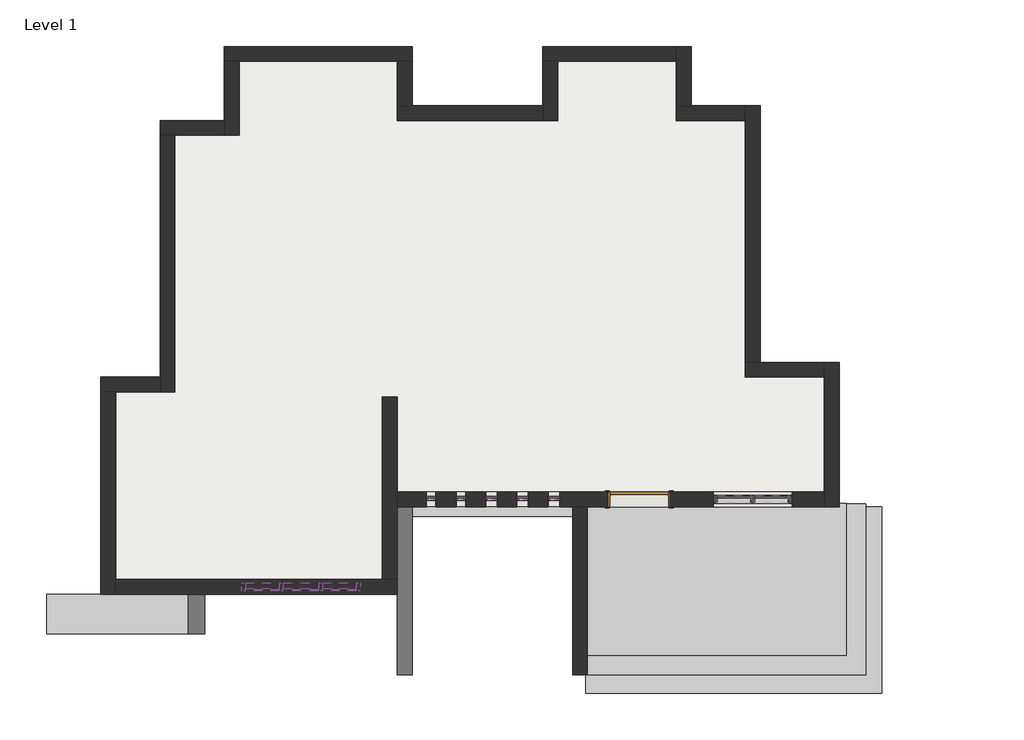
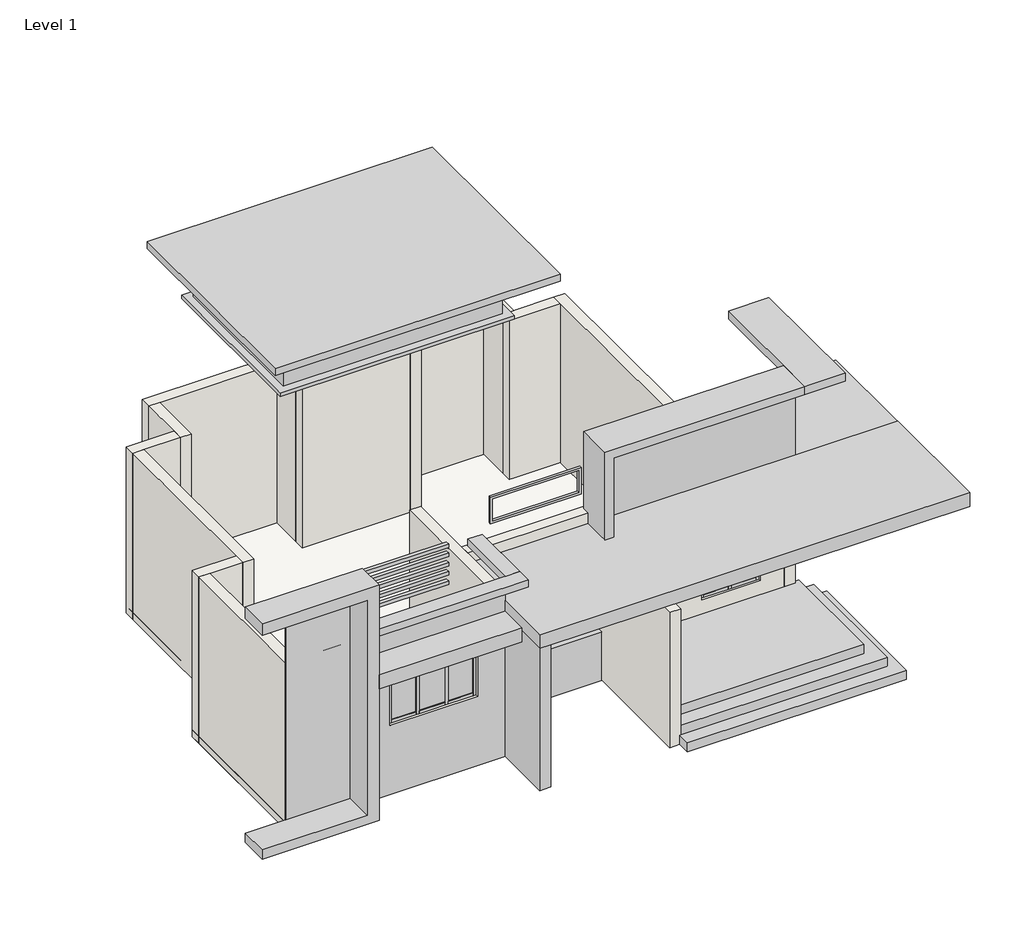
# One storey: 37 members, 19 walls, 10 plates, 1 door, 1 proxy, 1 slab.
"""IFC4 building model written with IfcOpenShell, lengths in millimetres."""

from ifc_helpers import new_model, si_unit, origin, origin_with_axes, place, context, project, spatial, polyline, outline, extrude, faceted_brep, transform, mapped, element, save
from components import generic_models_1_generic_models_1_dd7d6be2, door_e6f20f03, member_d2c643f7, member_0682bd88, member_4ec4fa50, member_0b7646a3, member_2b49869a, member_a980948f, member_75074519, member_d60e8053, member_2fae0574, system_panel_glazed_29dc7863, system_panel_glazed_ebf67a72, system_panel_glazed_1715a493, system_panel_glazed_fcede64b, system_panel_glazed_078fe0dd

model = new_model("IFC4")

# Units and contexts
model_context = context("Model", 3, world=origin())
ifc_project = project(units=[si_unit("LENGTHUNIT", "METRE", prefix="MILLI")], contexts=[model_context])

# Site, building, storey
site = spatial("IfcSite", under=ifc_project)
building = spatial("IfcBuilding", under=site)
storey = spatial("IfcBuildingStorey", under=building, Name="Level 1", Elevation=0.0)

# Proxy
placement = place(None, origin())
generic_models_1_generic_models_1_shape = generic_models_1_generic_models_1_dd7d6be2(model_context)
element("IfcBuildingElementProxy", 1, Name="Generic Models 1 : Generic Models 1", ObjectType="Generic Models 1 : Generic Models 1", at=placement, inside=storey, context=model_context, shape_type="MappedRepresentation", body=[
    mapped(generic_models_1_generic_models_1_shape, transform((0.0, 0.0, 0.0), x_axis=(1.0, 0.0, 0.0), y_axis=(0.0, 1.0, 0.0), z_axis=(0.0, 0.0, 1.0))),
])

# Door
door_shape = door_e6f20f03(model_context)
element("IfcDoor", 2, ObjectType="Door-Interior-Single-5_Panel_Vert-Wood : 3'6\" x 7'", at=placement, inside=storey, context=model_context, shape_type="MappedRepresentation", body=[
    mapped(door_shape, transform((1178.8071977, 2200.0207931, 609.6), x_axis=(-1.0, 0.0, 0.0), y_axis=(0.0, -1.0, 0.0), z_axis=(0.0, 0.0, 1.0))),
])

# Members
member_shape = member_d2c643f7(model_context)
element("IfcMember", 3, ObjectType="Rectangular Mullion : 1\" Square", at=placement, inside=storey, context=model_context, shape_type="MappedRepresentation", body=[
    mapped(member_shape, transform((-1983.4928023, 2196.8457931, 2975.2644013), x_axis=(0.0, 0.0, 1.0), y_axis=(0.0, -1.0, 0.0), z_axis=(1.0, 0.0, 0.0))),
])
element("IfcMember", 4, ObjectType="Rectangular Mullion : 1\" Square", at=placement, inside=storey, context=model_context, shape_type="MappedRepresentation", body=[
    mapped(member_shape, transform((-1519.9428023, 2196.8457931, 2975.2644013), x_axis=(0.0, 0.0, 1.0), y_axis=(0.0, -1.0, 0.0), z_axis=(1.0, 0.0, 0.0))),
])
element("IfcMember", 5, ObjectType="Rectangular Mullion : 1\" Square", at=placement, inside=storey, context=model_context, shape_type="MappedRepresentation", body=[
    mapped(member_shape, transform((-2085.0928023, 2196.8457931, 914.4), x_axis=(0.0, 0.0, -1.0), y_axis=(0.0, -1.0, 0.0), z_axis=(-1.0, 0.0, 0.0))),
])
element("IfcMember", 6, ObjectType="Rectangular Mullion : 1\" Square", at=placement, inside=storey, context=model_context, shape_type="MappedRepresentation", body=[
    mapped(member_shape, transform((-1621.5428023, 2196.8457931, 914.4), x_axis=(0.0, 0.0, -1.0), y_axis=(0.0, -1.0, 0.0), z_axis=(-1.0, 0.0, 0.0))),
])
member_2_shape = member_0682bd88(model_context)
element("IfcMember", 7, ObjectType="Rectangular Mullion : 1\" Square", at=placement, inside=storey, context=model_context, shape_type="MappedRepresentation", body=[
    mapped(member_2_shape, transform((-2110.4928023, 2196.8457931, 2975.2644013), x_axis=(-1.0, 0.0, 0.0), y_axis=(0.0, -1.0, 0.0), z_axis=(0.0, 0.0, 1.0))),
])
element("IfcMember", 8, ObjectType="Rectangular Mullion : 1\" Square", at=placement, inside=storey, context=model_context, shape_type="MappedRepresentation", body=[
    mapped(member_2_shape, transform((-1646.9428023, 2196.8457931, 2975.2644013), x_axis=(-1.0, 0.0, 0.0), y_axis=(0.0, -1.0, 0.0), z_axis=(0.0, 0.0, 1.0))),
])
element("IfcMember", 9, ObjectType="Rectangular Mullion : 1\" Square", at=placement, inside=storey, context=model_context, shape_type="MappedRepresentation", body=[
    mapped(member_2_shape, transform((-1189.7428023, 2196.8457931, 2975.2644013), x_axis=(-1.0, 0.0, 0.0), y_axis=(0.0, -1.0, 0.0), z_axis=(0.0, 0.0, 1.0))),
])
element("IfcMember", 10, ObjectType="Rectangular Mullion : 1\" Square", at=placement, inside=storey, context=model_context, shape_type="MappedRepresentation", body=[
    mapped(member_2_shape, transform((-707.1428023, 2196.8457931, 2975.2644013), x_axis=(-1.0, 0.0, 0.0), y_axis=(0.0, -1.0, 0.0), z_axis=(0.0, 0.0, 1.0))),
])
element("IfcMember", 11, ObjectType="Rectangular Mullion : 1\" Square", at=placement, inside=storey, context=model_context, shape_type="MappedRepresentation", body=[
    mapped(member_2_shape, transform((-224.5428023, 2196.8457931, 2975.2644013), x_axis=(-1.0, 0.0, 0.0), y_axis=(0.0, -1.0, 0.0), z_axis=(0.0, 0.0, 1.0))),
])
element("IfcMember", 12, ObjectType="Rectangular Mullion : 1\" Square", at=placement, inside=storey, context=model_context, shape_type="MappedRepresentation", body=[
    mapped(member_2_shape, transform((-1958.0928023, 2196.8457931, 914.4), x_axis=(1.0, 0.0, 0.0), y_axis=(0.0, -1.0, 0.0), z_axis=(0.0, 0.0, -1.0))),
])
element("IfcMember", 13, ObjectType="Rectangular Mullion : 1\" Square", at=placement, inside=storey, context=model_context, shape_type="MappedRepresentation", body=[
    mapped(member_2_shape, transform((-1494.5428023, 2196.8457931, 914.4), x_axis=(1.0, 0.0, 0.0), y_axis=(0.0, -1.0, 0.0), z_axis=(0.0, 0.0, -1.0))),
])
element("IfcMember", 14, ObjectType="Rectangular Mullion : 1\" Square", at=placement, inside=storey, context=model_context, shape_type="MappedRepresentation", body=[
    mapped(member_2_shape, transform((-1011.9428023, 2196.8457931, 914.4), x_axis=(1.0, 0.0, 0.0), y_axis=(0.0, -1.0, 0.0), z_axis=(0.0, 0.0, -1.0))),
])
element("IfcMember", 15, ObjectType="Rectangular Mullion : 1\" Square", at=placement, inside=storey, context=model_context, shape_type="MappedRepresentation", body=[
    mapped(member_2_shape, transform((-529.3428023, 2196.8457931, 914.4), x_axis=(1.0, 0.0, 0.0), y_axis=(0.0, -1.0, 0.0), z_axis=(0.0, 0.0, -1.0))),
])
element("IfcMember", 16, ObjectType="Rectangular Mullion : 1\" Square", at=placement, inside=storey, context=model_context, shape_type="MappedRepresentation", body=[
    mapped(member_2_shape, transform((-46.7428023, 2196.8457931, 914.4), x_axis=(1.0, 0.0, 0.0), y_axis=(0.0, -1.0, 0.0), z_axis=(0.0, 0.0, -1.0))),
])
member_3_shape = member_4ec4fa50(model_context)
element("IfcMember", 17, ObjectType="Rectangular Mullion : 1\" Square", at=placement, inside=storey, context=model_context, shape_type="MappedRepresentation", body=[
    mapped(member_3_shape, transform((-1037.3428023, 2196.8457931, 2975.2644013), x_axis=(0.0, 0.0, 1.0), y_axis=(0.0, -1.0, 0.0), z_axis=(1.0, 0.0, 0.0))),
])
element("IfcMember", 18, ObjectType="Rectangular Mullion : 1\" Square", at=placement, inside=storey, context=model_context, shape_type="MappedRepresentation", body=[
    mapped(member_3_shape, transform((-554.7428023, 2196.8457931, 2975.2644013), x_axis=(0.0, 0.0, 1.0), y_axis=(0.0, -1.0, 0.0), z_axis=(1.0, 0.0, 0.0))),
])
element("IfcMember", 19, ObjectType="Rectangular Mullion : 1\" Square", at=placement, inside=storey, context=model_context, shape_type="MappedRepresentation", body=[
    mapped(member_3_shape, transform((-72.1428023, 2196.8457931, 2975.2644013), x_axis=(0.0, 0.0, 1.0), y_axis=(0.0, -1.0, 0.0), z_axis=(1.0, 0.0, 0.0))),
])
element("IfcMember", 20, ObjectType="Rectangular Mullion : 1\" Square", at=placement, inside=storey, context=model_context, shape_type="MappedRepresentation", body=[
    mapped(member_3_shape, transform((-1164.3428023, 2196.8457931, 914.4), x_axis=(0.0, 0.0, -1.0), y_axis=(0.0, -1.0, 0.0), z_axis=(-1.0, 0.0, 0.0))),
])
element("IfcMember", 21, ObjectType="Rectangular Mullion : 1\" Square", at=placement, inside=storey, context=model_context, shape_type="MappedRepresentation", body=[
    mapped(member_3_shape, transform((-681.7428023, 2196.8457931, 914.4), x_axis=(0.0, 0.0, -1.0), y_axis=(0.0, -1.0, 0.0), z_axis=(-1.0, 0.0, 0.0))),
])
element("IfcMember", 22, ObjectType="Rectangular Mullion : 1\" Square", at=placement, inside=storey, context=model_context, shape_type="MappedRepresentation", body=[
    mapped(member_3_shape, transform((-199.1428023, 2196.8457931, 914.4), x_axis=(0.0, 0.0, -1.0), y_axis=(0.0, -1.0, 0.0), z_axis=(-1.0, 0.0, 0.0))),
])
member_4_shape = member_0b7646a3(model_context)
element("IfcMember", 23, ObjectType="Rectangular Mullion : 2.5\" x 5\" rectangular", at=placement, inside=storey, context=model_context, shape_type="MappedRepresentation", body=[
    mapped(member_4_shape, transform((-4891.7928023, 844.2957931, 2743.2), x_axis=(0.0, 0.0, 1.0), y_axis=(0.0, 1.0, 0.0), z_axis=(-1.0, 0.0, 0.0))),
])
element("IfcMember", 24, ObjectType="Rectangular Mullion : 2.5\" x 5\" rectangular", at=placement, inside=storey, context=model_context, shape_type="MappedRepresentation", body=[
    mapped(member_4_shape, transform((-3704.3428023, 844.2957931, 2743.2), x_axis=(0.0, 0.0, 1.0), y_axis=(0.0, 1.0, 0.0), z_axis=(-1.0, 0.0, 0.0))),
])
element("IfcMember", 25, ObjectType="Rectangular Mullion : 2.5\" x 5\" rectangular", at=placement, inside=storey, context=model_context, shape_type="MappedRepresentation", body=[
    mapped(member_4_shape, transform((3477.5071977, 2196.8457931, 2743.2), x_axis=(0.0, 0.0, 1.0), y_axis=(0.0, -1.0, 0.0), z_axis=(1.0, 0.0, 0.0))),
])
element("IfcMember", 26, ObjectType="Rectangular Mullion : 2.5\" x 5\" rectangular", at=placement, inside=storey, context=model_context, shape_type="MappedRepresentation", body=[
    mapped(member_4_shape, transform((2899.6571977, 2196.8457931, 2743.2), x_axis=(0.0, 0.0, 1.0), y_axis=(0.0, -1.0, 0.0), z_axis=(1.0, 0.0, 0.0))),
])
element("IfcMember", 27, ObjectType="Rectangular Mullion : 2.5\" x 5\" rectangular", at=placement, inside=storey, context=model_context, shape_type="MappedRepresentation", body=[
    mapped(member_4_shape, transform((-3189.9928023, 844.2957931, 1524.0), x_axis=(0.0, 0.0, -1.0), y_axis=(0.0, 1.0, 0.0), z_axis=(1.0, 0.0, 0.0))),
])
element("IfcMember", 28, ObjectType="Rectangular Mullion : 2.5\" x 5\" rectangular", at=placement, inside=storey, context=model_context, shape_type="MappedRepresentation", body=[
    mapped(member_4_shape, transform((-4377.4428023, 844.2957931, 1524.0), x_axis=(0.0, 0.0, -1.0), y_axis=(0.0, 1.0, 0.0), z_axis=(1.0, 0.0, 0.0))),
])
element("IfcMember", 29, ObjectType="Rectangular Mullion : 2.5\" x 5\" rectangular", at=placement, inside=storey, context=model_context, shape_type="MappedRepresentation", body=[
    mapped(member_4_shape, transform((2385.3071977, 2196.8457931, 914.4), x_axis=(0.0, 0.0, -1.0), y_axis=(0.0, -1.0, 0.0), z_axis=(-1.0, 0.0, 0.0))),
])
element("IfcMember", 30, ObjectType="Rectangular Mullion : 2.5\" x 5\" rectangular", at=placement, inside=storey, context=model_context, shape_type="MappedRepresentation", body=[
    mapped(member_4_shape, transform((2963.1571977, 2196.8457931, 914.4), x_axis=(0.0, 0.0, -1.0), y_axis=(0.0, -1.0, 0.0), z_axis=(-1.0, 0.0, 0.0))),
])
member_5_shape = member_2b49869a(model_context)
element("IfcMember", 31, ObjectType="Rectangular Mullion : 2.5\" x 5\" rectangular", at=placement, inside=storey, context=model_context, shape_type="MappedRepresentation", body=[
    mapped(member_5_shape, transform((-4345.6928023, 844.2957931, 1524.0), x_axis=(-1.0, 0.0, 0.0), y_axis=(0.0, 1.0, 0.0), z_axis=(0.0, 0.0, -1.0))),
])
element("IfcMember", 32, ObjectType="Rectangular Mullion : 2.5\" x 5\" rectangular", at=placement, inside=storey, context=model_context, shape_type="MappedRepresentation", body=[
    mapped(member_5_shape, transform((-3736.0928023, 844.2957931, 1524.0), x_axis=(-1.0, 0.0, 0.0), y_axis=(0.0, 1.0, 0.0), z_axis=(0.0, 0.0, -1.0))),
])
member_6_shape = member_a980948f(model_context)
element("IfcMember", 33, ObjectType="Rectangular Mullion : 2.5\" x 5\" rectangular", at=placement, inside=storey, context=model_context, shape_type="MappedRepresentation", body=[
    mapped(member_6_shape, transform((-3767.8428023, 844.2957931, 1524.0), x_axis=(0.0, 0.0, -1.0), y_axis=(0.0, 1.0, 0.0), z_axis=(1.0, 0.0, 0.0))),
])
element("IfcMember", 34, ObjectType="Rectangular Mullion : 2.5\" x 5\" rectangular", at=placement, inside=storey, context=model_context, shape_type="MappedRepresentation", body=[
    mapped(member_6_shape, transform((-4313.9428023, 844.2957931, 2743.2), x_axis=(0.0, 0.0, 1.0), y_axis=(0.0, 1.0, 0.0), z_axis=(-1.0, 0.0, 0.0))),
])
member_7_shape = member_75074519(model_context)
element("IfcMember", 35, ObjectType="Rectangular Mullion : 2.5\" x 5\" rectangular", at=placement, inside=storey, context=model_context, shape_type="MappedRepresentation", body=[
    mapped(member_7_shape, transform((-3126.4928023, 844.2957931, 2743.2), x_axis=(1.0, 0.0, 0.0), y_axis=(0.0, 1.0, 0.0), z_axis=(0.0, 0.0, 1.0))),
])
element("IfcMember", 36, ObjectType="Rectangular Mullion : 2.5\" x 5\" rectangular", at=placement, inside=storey, context=model_context, shape_type="MappedRepresentation", body=[
    mapped(member_7_shape, transform((-4955.2928023, 844.2957931, 1524.0), x_axis=(-1.0, 0.0, 0.0), y_axis=(0.0, 1.0, 0.0), z_axis=(0.0, 0.0, -1.0))),
])
member_8_shape = member_d60e8053(model_context)
element("IfcMember", 37, ObjectType="Rectangular Mullion : 2.5\" x 5\" rectangular", at=placement, inside=storey, context=model_context, shape_type="MappedRepresentation", body=[
    mapped(member_8_shape, transform((2931.4071977, 2196.8457931, 914.4), x_axis=(1.0, 0.0, 0.0), y_axis=(0.0, -1.0, 0.0), z_axis=(0.0, 0.0, -1.0))),
])
member_9_shape = member_2fae0574(model_context)
element("IfcMember", 38, ObjectType="Rectangular Mullion : 2.5\" x 5\" rectangular", at=placement, inside=storey, context=model_context, shape_type="MappedRepresentation", body=[
    mapped(member_9_shape, transform((2321.8071977, 2196.8457931, 2743.2), x_axis=(-1.0, 0.0, 0.0), y_axis=(0.0, -1.0, 0.0), z_axis=(0.0, 0.0, 1.0))),
])
element("IfcMember", 39, ObjectType="Rectangular Mullion : 2.5\" x 5\" rectangular", at=placement, inside=storey, context=model_context, shape_type="MappedRepresentation", body=[
    mapped(member_9_shape, transform((3541.0071977, 2196.8457931, 914.4), x_axis=(1.0, 0.0, 0.0), y_axis=(0.0, -1.0, 0.0), z_axis=(0.0, 0.0, -1.0))),
])

# Plates
system_panel_glazed_shape = system_panel_glazed_29dc7863(model_context)
element("IfcPlate", 40, ObjectType="System Panel : Glazed", at=placement, inside=storey, context=model_context, shape_type="MappedRepresentation", body=[
    mapped(system_panel_glazed_shape, transform((-2034.2928023, 2196.8457931, 914.4), x_axis=(1.0, 0.0, 0.0), y_axis=(0.0, 1.0, 0.0), z_axis=(0.0, 0.0, 1.0))),
])
element("IfcPlate", 41, ObjectType="System Panel : Glazed", at=placement, inside=storey, context=model_context, shape_type="MappedRepresentation", body=[
    mapped(system_panel_glazed_shape, transform((-1570.7428023, 2196.8457931, 914.4), x_axis=(1.0, 0.0, 0.0), y_axis=(0.0, 1.0, 0.0), z_axis=(0.0, 0.0, 1.0))),
])
system_panel_glazed_2_shape = system_panel_glazed_ebf67a72(model_context)
element("IfcPlate", 42, ObjectType="System Panel : Glazed", at=placement, inside=storey, context=model_context, shape_type="MappedRepresentation", body=[
    mapped(system_panel_glazed_2_shape, transform((-1100.8428023, 2196.8457931, 914.4), x_axis=(1.0, 0.0, 0.0), y_axis=(0.0, 1.0, 0.0), z_axis=(0.0, 0.0, 1.0))),
])
element("IfcPlate", 43, ObjectType="System Panel : Glazed", at=placement, inside=storey, context=model_context, shape_type="MappedRepresentation", body=[
    mapped(system_panel_glazed_2_shape, transform((-618.2428023, 2196.8457931, 914.4), x_axis=(1.0, 0.0, 0.0), y_axis=(0.0, 1.0, 0.0), z_axis=(0.0, 0.0, 1.0))),
])
element("IfcPlate", 44, ObjectType="System Panel : Glazed", at=placement, inside=storey, context=model_context, shape_type="MappedRepresentation", body=[
    mapped(system_panel_glazed_2_shape, transform((-135.6428023, 2196.8457931, 914.4), x_axis=(1.0, 0.0, 0.0), y_axis=(0.0, 1.0, 0.0), z_axis=(0.0, 0.0, 1.0))),
])
system_panel_glazed_3_shape = system_panel_glazed_1715a493(model_context)
element("IfcPlate", 45, ObjectType="System Panel : Glazed", at=placement, inside=storey, context=model_context, shape_type="MappedRepresentation", body=[
    mapped(system_panel_glazed_3_shape, transform((-3447.1678023, 844.2957931, 1587.5), x_axis=(-1.0, 0.0, 0.0), y_axis=(0.0, -1.0, 0.0), z_axis=(0.0, 0.0, 1.0))),
])
element("IfcPlate", 46, ObjectType="System Panel : Glazed", at=placement, inside=storey, context=model_context, shape_type="MappedRepresentation", body=[
    mapped(system_panel_glazed_3_shape, transform((-4634.6178023, 844.2957931, 1587.5), x_axis=(-1.0, 0.0, 0.0), y_axis=(0.0, -1.0, 0.0), z_axis=(0.0, 0.0, 1.0))),
])
system_panel_glazed_4_shape = system_panel_glazed_fcede64b(model_context)
element("IfcPlate", 47, ObjectType="System Panel : Glazed", at=placement, inside=storey, context=model_context, shape_type="MappedRepresentation", body=[
    mapped(system_panel_glazed_4_shape, transform((-4040.8928023, 844.2957931, 1587.5), x_axis=(-1.0, 0.0, 0.0), y_axis=(0.0, -1.0, 0.0), z_axis=(0.0, 0.0, 1.0))),
])
system_panel_glazed_5_shape = system_panel_glazed_078fe0dd(model_context)
element("IfcPlate", 48, ObjectType="System Panel : Glazed", at=placement, inside=storey, context=model_context, shape_type="MappedRepresentation", body=[
    mapped(system_panel_glazed_5_shape, transform((2642.4821977, 2196.8457931, 977.9), x_axis=(1.0, 0.0, 0.0), y_axis=(0.0, 1.0, 0.0), z_axis=(0.0, 0.0, 1.0))),
])
element("IfcPlate", 49, ObjectType="System Panel : Glazed", at=placement, inside=storey, context=model_context, shape_type="MappedRepresentation", body=[
    mapped(system_panel_glazed_5_shape, transform((3220.3321977, 2196.8457931, 977.9), x_axis=(1.0, 0.0, 0.0), y_axis=(0.0, 1.0, 0.0), z_axis=(0.0, 0.0, 1.0))),
])

# Slab
element("IfcSlab", 50, ObjectType="6\" floor", at=placement, inside=storey, context=model_context, shape_type="SweptSolid", body=[
    extrude(outline(polyline([(-5221.9928023, 9188.1957931), (-2326.3928023, 9188.1957931), (-2326.3928023, 8273.7957931), (-307.0928023, 8273.7957931), (-307.0928023, 9188.1957931), (1978.9071977, 9188.1957931), (1978.9071977, 8273.7957931), (3045.7071977, 8273.7957931), (3045.7071977, 4311.3957931), (4264.9071977, 4311.3957931), (4264.9071977, 2082.5457931), (150.1071977, 2082.5457931), (-2554.9928023, 2082.5457931), (-2554.9928023, 729.9957931), (-7126.9928023, 729.9957931), (-7126.9928023, 4082.7957931), (-6212.5928023, 4082.7957931), (-6212.5928023, 8045.1957931), (-5221.9928023, 8045.1957931), (-5221.9928023, 9188.1957931)])), origin_with_axes(), (0.0, 0.0, 1.0), 152.4),
])

# Walls
element("IfcWall", 51, ObjectType="9\" wall", at=placement, inside=storey, context=model_context, shape_type="Brep", body=[
    faceted_brep([(-2326.3928023, 9188.1957931, 0.0), (-5221.9928023, 9188.1957931, 0.0), (-5221.9928023, 9188.1957931, 3657.6), (-2326.3928023, 9188.1957931, 3657.6), (-2326.3928023, 8959.5957931, 0.0), (-2326.3928023, 8959.5957931, 3657.6), (-2554.9928023, 8959.5957931, 3657.6), (-4993.3928023, 8959.5957931, 3657.6), (-5221.9928023, 8959.5957931, 3657.6), (-5221.9928023, 8959.5957931, 0.0), (-4993.3928023, 8959.5957931, 0.0), (-2554.9928023, 8959.5957931, 0.0)], [[[0, 1, 2, 3]], [[4, 5, 6, 7, 8, 9, 10, 11]], [[1, 0, 4, 11, 10, 9]], [[3, 2, 8, 7, 6, 5]], [[2, 1, 9, 8]], [[0, 3, 5, 4]]]),
])
element("IfcWall", 52, ObjectType="9\" wall", at=placement, inside=storey, context=model_context, shape_type="Brep", body=[
    faceted_brep([(-5221.9928023, 8959.5957931, 0.0), (-5221.9928023, 8045.1957931, 0.0), (-5221.9928023, 7816.5957931, 0.0), (-5221.9928023, 7816.5957931, 3657.6), (-5221.9928023, 8045.1957931, 3657.6), (-5221.9928023, 8959.5957931, 3657.6), (-4993.3928023, 8959.5957931, 0.0), (-4993.3928023, 8959.5957931, 3657.6), (-4993.3928023, 7816.5957931, 3657.6), (-4993.3928023, 7816.5957931, 0.0)], [[[0, 1, 2, 3, 4, 5]], [[6, 7, 8, 9]], [[2, 1, 0, 6, 9]], [[5, 4, 3, 8, 7]], [[0, 5, 7, 6]], [[3, 2, 9, 8]]]),
])
element("IfcWall", 53, ObjectType="9\" wall", at=placement, inside=storey, context=model_context, shape_type="Brep", body=[
    faceted_brep([(-5221.9928023, 8045.1957931, 0.0), (-6212.5928023, 8045.1957931, 0.0), (-6212.5928023, 8045.1957931, 3657.6), (-5221.9928023, 8045.1957931, 3657.6), (-5221.9928023, 7816.5957931, 0.0), (-5221.9928023, 7816.5957931, 3657.6), (-5983.9928023, 7816.5957931, 3657.6), (-6212.5928023, 7816.5957931, 3657.6), (-6212.5928023, 7816.5957931, 0.0), (-5983.9928023, 7816.5957931, 0.0)], [[[0, 1, 2, 3]], [[4, 5, 6, 7, 8, 9]], [[1, 0, 4, 9, 8]], [[3, 2, 7, 6, 5]], [[0, 3, 5, 4]], [[2, 1, 8, 7]]]),
])
element("IfcWall", 54, ObjectType="9\" wall", at=placement, inside=storey, context=model_context, shape_type="Brep", body=[
    faceted_brep([(-6212.5928023, 7816.5957931, 0.0), (-6212.5928023, 4082.7957931, 0.0), (-6212.5928023, 3854.1957931, 0.0), (-6212.5928023, 3854.1957931, 3657.6), (-6212.5928023, 4082.7957931, 3657.6), (-6212.5928023, 7816.5957931, 3657.6), (-5983.9928023, 7816.5957931, 0.0), (-5983.9928023, 7816.5957931, 3657.6), (-5983.9928023, 3854.1957931, 3657.6), (-5983.9928023, 3854.1957931, 0.0)], [[[0, 1, 2, 3, 4, 5]], [[6, 7, 8, 9]], [[2, 1, 0, 6, 9]], [[5, 4, 3, 8, 7]], [[0, 5, 7, 6]], [[3, 2, 9, 8]]]),
])
element("IfcWall", 55, ObjectType="9\" wall", at=placement, inside=storey, context=model_context, shape_type="Brep", body=[
    faceted_brep([(-6212.5928023, 4082.7957931, 0.0), (-7126.9928023, 4082.7957931, 0.0), (-7126.9928023, 4082.7957931, 3657.6), (-6212.5928023, 4082.7957931, 3657.6), (-6212.5928023, 3854.1957931, 0.0), (-6212.5928023, 3854.1957931, 3657.6), (-6898.3928023, 3854.1957931, 3657.6), (-7126.9928023, 3854.1957931, 3657.6), (-7126.9928023, 3854.1957931, 0.0), (-6898.3928023, 3854.1957931, 0.0)], [[[0, 1, 2, 3]], [[4, 5, 6, 7, 8, 9]], [[1, 0, 4, 9, 8]], [[3, 2, 7, 6, 5]], [[0, 3, 5, 4]], [[2, 1, 8, 7]]]),
])
element("IfcWall", 56, ObjectType="9\" wall", at=placement, inside=storey, context=model_context, shape_type="Brep", body=[
    faceted_brep([(-7126.9928023, 3854.1957931, 0.0), (-7126.9928023, 729.9957931, 0.0), (-7126.9928023, 729.9957931, 3657.6), (-7126.9928023, 3854.1957931, 3657.6), (-6898.3928023, 3854.1957931, 0.0), (-6898.3928023, 3854.1957931, 3657.6), (-6898.3928023, 958.5957931, 3657.6), (-6898.3928023, 729.9957931, 3657.6), (-6898.3928023, 729.9957931, 0.0), (-6898.3928023, 958.5957931, 0.0)], [[[0, 1, 2, 3]], [[4, 5, 6, 7, 8, 9]], [[1, 0, 4, 9, 8]], [[3, 2, 7, 6, 5]], [[0, 3, 5, 4]], [[2, 1, 8, 7]]]),
])
element("IfcWall", 57, ObjectType="9\" wall", at=placement, inside=storey, context=model_context, shape_type="Brep", body=[
    faceted_brep([(-6898.3928023, 729.9957931, 0.0), (-2554.9928023, 729.9957931, 0.0), (-2554.9928023, 729.9957931, 3657.6), (-6898.3928023, 729.9957931, 3657.6), (-3126.4928023, 729.9957931, 2743.2), (-3126.4928023, 729.9957931, 1524.0), (-4955.2928023, 729.9957931, 1524.0), (-4955.2928023, 729.9957931, 2743.2), (-2554.9928023, 958.5957931, 0.0), (-2783.5928023, 958.5957931, 0.0), (-6898.3928023, 958.5957931, 0.0), (-6898.3928023, 958.5957931, 3657.6), (-2783.5928023, 958.5957931, 3657.6), (-2554.9928023, 958.5957931, 3657.6), (-3126.4928023, 958.5957931, 1524.0), (-3126.4928023, 958.5957931, 2743.2), (-4955.2928023, 958.5957931, 2743.2), (-4955.2928023, 958.5957931, 1524.0)], [[[0, 1, 2, 3], [4, 5, 6, 7]], [[8, 9, 10, 11, 12, 13], [14, 15, 16, 17]], [[1, 0, 10, 9, 8]], [[3, 2, 13, 12, 11]], [[0, 3, 11, 10]], [[2, 1, 8, 13]], [[14, 5, 4, 15]], [[15, 4, 7, 16]], [[16, 7, 6, 17]], [[5, 14, 17, 6]]]),
])
element("IfcWall", 58, ObjectType="9\" wall", at=placement, inside=storey, context=model_context, shape_type="Brep", body=[
    faceted_brep([(-2554.9928023, 958.5957931, 0.0), (-2554.9928023, 2082.5457931, 0.0), (-2554.9928023, 2311.1457931, 0.0), (-2554.9928023, 3777.9957931, 0.0), (-2554.9928023, 3777.9957931, 3657.6), (-2554.9928023, 2311.1457931, 3657.6), (-2554.9928023, 2082.5457931, 3657.6), (-2554.9928023, 958.5957931, 3657.6), (-2783.5928023, 958.5957931, 0.0), (-2783.5928023, 958.5957931, 3657.6), (-2783.5928023, 3777.9957931, 3657.6), (-2783.5928023, 3777.9957931, 0.0)], [[[0, 1, 2, 3, 4, 5, 6, 7]], [[8, 9, 10, 11]], [[3, 2, 1, 0, 8, 11]], [[4, 3, 11, 10]], [[7, 6, 5, 4, 10, 9]], [[0, 7, 9, 8]]]),
])
element("IfcWall", 59, ObjectType="9\" wall", at=placement, inside=storey, context=model_context, shape_type="Brep", body=[
    faceted_brep([(-2554.9928023, 2082.5457931, 0.0), (150.1071977, 2082.5457931, 0.0), (378.7071977, 2082.5457931, 0.0), (4036.3071977, 2082.5457931, 0.0), (4036.3071977, 2082.5457931, 3657.6), (-2554.9928023, 2082.5457931, 3657.6), (696.2071977, 2082.5457931, 609.6), (696.2071977, 2082.5457931, 2768.6), (1661.4071977, 2082.5457931, 2768.6), (1661.4071977, 2082.5457931, 609.6), (2321.8071977, 2082.5457931, 914.4), (2321.8071977, 2082.5457931, 2743.2), (3541.0071977, 2082.5457931, 2743.2), (3541.0071977, 2082.5457931, 914.4), (-2110.4928023, 2082.5457931, 914.4), (-2110.4928023, 2082.5457931, 2975.2644013), (-1958.0928023, 2082.5457931, 2975.2644013), (-1958.0928023, 2082.5457931, 914.4), (-1646.9428023, 2082.5457931, 914.4), (-1646.9428023, 2082.5457931, 2975.2644013), (-1494.5428023, 2082.5457931, 2975.2644013), (-1494.5428023, 2082.5457931, 914.4), (-1189.7428023, 2082.5457931, 914.4), (-1189.7428023, 2082.5457931, 2975.2644013), (-1011.9428023, 2082.5457931, 2975.2644013), (-1011.9428023, 2082.5457931, 914.4), (-707.1428023, 2082.5457931, 914.4), (-707.1428023, 2082.5457931, 2975.2644013), (-529.3428023, 2082.5457931, 2975.2644013), (-529.3428023, 2082.5457931, 914.4), (-224.5428023, 2082.5457931, 914.4), (-224.5428023, 2082.5457931, 2975.2644013), (-46.7428023, 2082.5457931, 2975.2644013), (-46.7428023, 2082.5457931, 914.4), (4036.3071977, 2311.1457931, 0.0), (-2554.9928023, 2311.1457931, 0.0), (-2554.9928023, 2311.1457931, 3657.6), (4036.3071977, 2311.1457931, 3657.6), (696.2071977, 2311.1457931, 2768.6), (696.2071977, 2311.1457931, 609.6), (1661.4071977, 2311.1457931, 609.6), (1661.4071977, 2311.1457931, 2768.6), (2321.8071977, 2311.1457931, 2743.2), (2321.8071977, 2311.1457931, 914.4), (3541.0071977, 2311.1457931, 914.4), (3541.0071977, 2311.1457931, 2743.2), (-2110.4928023, 2311.1457931, 2975.2644013), (-2110.4928023, 2311.1457931, 914.4), (-1958.0928023, 2311.1457931, 914.4), (-1958.0928023, 2311.1457931, 2975.2644013), (-1646.9428023, 2311.1457931, 2975.2644013), (-1646.9428023, 2311.1457931, 914.4), (-1494.5428023, 2311.1457931, 914.4), (-1494.5428023, 2311.1457931, 2975.2644013), (-1189.7428023, 2311.1457931, 2975.2644013), (-1189.7428023, 2311.1457931, 914.4), (-1011.9428023, 2311.1457931, 914.4), (-1011.9428023, 2311.1457931, 2975.2644013), (-707.1428023, 2311.1457931, 2975.2644013), (-707.1428023, 2311.1457931, 914.4), (-529.3428023, 2311.1457931, 914.4), (-529.3428023, 2311.1457931, 2975.2644013), (-224.5428023, 2311.1457931, 2975.2644013), (-224.5428023, 2311.1457931, 914.4), (-46.7428023, 2311.1457931, 914.4), (-46.7428023, 2311.1457931, 2975.2644013)], [[[0, 1, 2, 3, 4, 5], [6, 7, 8, 9], [10, 11, 12, 13], [14, 15, 16, 17], [18, 19, 20, 21], [22, 23, 24, 25], [26, 27, 28, 29], [30, 31, 32, 33]], [[34, 35, 36, 37], [38, 39, 40, 41], [42, 43, 44, 45], [46, 47, 48, 49], [50, 51, 52, 53], [54, 55, 56, 57], [58, 59, 60, 61], [62, 63, 64, 65]], [[3, 2, 1, 0, 35, 34]], [[5, 4, 37, 36]], [[0, 5, 36, 35]], [[4, 3, 34, 37]], [[6, 39, 38, 7]], [[7, 38, 41, 8]], [[40, 9, 8, 41]], [[39, 6, 9, 40]], [[42, 11, 10, 43]], [[11, 42, 45, 12]], [[12, 45, 44, 13]], [[43, 10, 13, 44]], [[14, 47, 46, 15]], [[15, 46, 49, 16]], [[48, 17, 16, 49]], [[47, 14, 17, 48]], [[18, 51, 50, 19]], [[19, 50, 53, 20]], [[52, 21, 20, 53]], [[51, 18, 21, 52]], [[22, 55, 54, 23]], [[23, 54, 57, 24]], [[56, 25, 24, 57]], [[55, 22, 25, 56]], [[26, 59, 58, 27]], [[27, 58, 61, 28]], [[60, 29, 28, 61]], [[59, 26, 29, 60]], [[30, 63, 62, 31]], [[31, 62, 65, 32]], [[32, 65, 64, 33]], [[63, 30, 33, 64]]]),
])
element("IfcWall", 60, ObjectType="9\" wall", at=placement, inside=storey, context=model_context, shape_type="SweptSolid", body=[
    extrude(outline(polyline([(150.1071977, -514.6042069), (150.1071977, 2082.5457931), (378.7071977, 2082.5457931), (378.7071977, -514.6042069), (150.1071977, -514.6042069)])), origin_with_axes(), (0.0, 0.0, 1.0), 2975.2644013),
])
element("IfcWall", 61, ObjectType="9\" wall", at=placement, inside=storey, context=model_context, shape_type="Brep", body=[
    faceted_brep([(4264.9071977, 2082.5457931, 0.0), (4264.9071977, 4311.3957931, 0.0), (4264.9071977, 4311.3957931, 3657.6), (4264.9071977, 2082.5457931, 3657.6), (4036.3071977, 2082.5457931, 0.0), (4036.3071977, 2082.5457931, 3657.6), (4036.3071977, 2311.1457931, 3657.6), (4036.3071977, 4082.7957931, 3657.6), (4036.3071977, 4311.3957931, 3657.6), (4036.3071977, 4311.3957931, 0.0), (4036.3071977, 4082.7957931, 0.0), (4036.3071977, 2311.1457931, 0.0)], [[[0, 1, 2, 3]], [[4, 5, 6, 7, 8, 9, 10, 11]], [[1, 0, 4, 11, 10, 9]], [[3, 2, 8, 7, 6, 5]], [[0, 3, 5, 4]], [[2, 1, 9, 8]]]),
])
element("IfcWall", 62, ObjectType="9\" wall", at=placement, inside=storey, context=model_context, shape_type="Brep", body=[
    faceted_brep([(4036.3071977, 4311.3957931, 0.0), (3045.7071977, 4311.3957931, 0.0), (2817.1071977, 4311.3957931, 0.0), (2817.1071977, 4311.3957931, 3657.6), (3045.7071977, 4311.3957931, 3657.6), (4036.3071977, 4311.3957931, 3657.6), (4036.3071977, 4082.7957931, 0.0), (4036.3071977, 4082.7957931, 3657.6), (2817.1071977, 4082.7957931, 3657.6), (2817.1071977, 4082.7957931, 0.0)], [[[0, 1, 2, 3, 4, 5]], [[6, 7, 8, 9]], [[2, 1, 0, 6, 9]], [[5, 4, 3, 8, 7]], [[0, 5, 7, 6]], [[3, 2, 9, 8]]]),
])
element("IfcWall", 63, ObjectType="9\" wall", at=placement, inside=storey, context=model_context, shape_type="Brep", body=[
    faceted_brep([(3045.7071977, 4311.3957931, 0.0), (3045.7071977, 8273.7957931, 0.0), (3045.7071977, 8273.7957931, 3657.6), (3045.7071977, 4311.3957931, 3657.6), (2817.1071977, 4311.3957931, 0.0), (2817.1071977, 4311.3957931, 3657.6), (2817.1071977, 8045.1957931, 3657.6), (2817.1071977, 8273.7957931, 3657.6), (2817.1071977, 8273.7957931, 0.0), (2817.1071977, 8045.1957931, 0.0)], [[[0, 1, 2, 3]], [[4, 5, 6, 7, 8, 9]], [[1, 0, 4, 9, 8]], [[3, 2, 7, 6, 5]], [[0, 3, 5, 4]], [[2, 1, 8, 7]]]),
])
element("IfcWall", 64, ObjectType="9\" wall", at=placement, inside=storey, context=model_context, shape_type="Brep", body=[
    faceted_brep([(2817.1071977, 8273.7957931, 0.0), (1978.9071977, 8273.7957931, 0.0), (1750.3071977, 8273.7957931, 0.0), (1750.3071977, 8273.7957931, 3657.6), (1978.9071977, 8273.7957931, 3657.6), (2817.1071977, 8273.7957931, 3657.6), (2817.1071977, 8045.1957931, 0.0), (2817.1071977, 8045.1957931, 3657.6), (1750.3071977, 8045.1957931, 3657.6), (1750.3071977, 8045.1957931, 0.0)], [[[0, 1, 2, 3, 4, 5]], [[6, 7, 8, 9]], [[2, 1, 0, 6, 9]], [[5, 4, 3, 8, 7]], [[0, 5, 7, 6]], [[3, 2, 9, 8]]]),
])
element("IfcWall", 65, ObjectType="9\" wall", at=placement, inside=storey, context=model_context, shape_type="Brep", body=[
    faceted_brep([(1978.9071977, 8273.7957931, 0.0), (1978.9071977, 9188.1957931, 0.0), (1978.9071977, 9188.1957931, 3657.6), (1978.9071977, 8273.7957931, 3657.6), (1750.3071977, 8273.7957931, 0.0), (1750.3071977, 8273.7957931, 3657.6), (1750.3071977, 8959.5957931, 3657.6), (1750.3071977, 9188.1957931, 3657.6), (1750.3071977, 9188.1957931, 0.0), (1750.3071977, 8959.5957931, 0.0)], [[[0, 1, 2, 3]], [[4, 5, 6, 7, 8, 9]], [[1, 0, 4, 9, 8]], [[3, 2, 7, 6, 5]], [[0, 3, 5, 4]], [[2, 1, 8, 7]]]),
])
element("IfcWall", 66, ObjectType="9\" wall", at=placement, inside=storey, context=model_context, shape_type="Brep", body=[
    faceted_brep([(1750.3071977, 9188.1957931, 0.0), (-307.0928023, 9188.1957931, 0.0), (-307.0928023, 9188.1957931, 3657.6), (1750.3071977, 9188.1957931, 3657.6), (1750.3071977, 8959.5957931, 0.0), (1750.3071977, 8959.5957931, 3657.6), (-78.4928023, 8959.5957931, 3657.6), (-307.0928023, 8959.5957931, 3657.6), (-307.0928023, 8959.5957931, 0.0), (-78.4928023, 8959.5957931, 0.0)], [[[0, 1, 2, 3]], [[4, 5, 6, 7, 8, 9]], [[1, 0, 4, 9, 8]], [[3, 2, 7, 6, 5]], [[0, 3, 5, 4]], [[2, 1, 8, 7]]]),
])
element("IfcWall", 67, ObjectType="9\" wall", at=placement, inside=storey, context=model_context, shape_type="Brep", body=[
    faceted_brep([(-307.0928023, 8959.5957931, 0.0), (-307.0928023, 8273.7957931, 0.0), (-307.0928023, 8045.1957931, 0.0), (-307.0928023, 8045.1957931, 3657.6), (-307.0928023, 8273.7957931, 3657.6), (-307.0928023, 8959.5957931, 3657.6), (-78.4928023, 8959.5957931, 0.0), (-78.4928023, 8959.5957931, 3657.6), (-78.4928023, 8045.1957931, 3657.6), (-78.4928023, 8045.1957931, 0.0)], [[[0, 1, 2, 3, 4, 5]], [[6, 7, 8, 9]], [[2, 1, 0, 6, 9]], [[5, 4, 3, 8, 7]], [[0, 5, 7, 6]], [[3, 2, 9, 8]]]),
])
element("IfcWall", 68, ObjectType="9\" wall", at=placement, inside=storey, context=model_context, shape_type="Brep", body=[
    faceted_brep([(-307.0928023, 8273.7957931, 0.0), (-2326.3928023, 8273.7957931, 0.0), (-2554.9928023, 8273.7957931, 0.0), (-2554.9928023, 8273.7957931, 3657.6), (-2326.3928023, 8273.7957931, 3657.6), (-307.0928023, 8273.7957931, 3657.6), (-307.0928023, 8045.1957931, 0.0), (-307.0928023, 8045.1957931, 3657.6), (-2554.9928023, 8045.1957931, 3657.6), (-2554.9928023, 8045.1957931, 0.0)], [[[0, 1, 2, 3, 4, 5]], [[6, 7, 8, 9]], [[2, 1, 0, 6, 9]], [[5, 4, 3, 8, 7]], [[0, 5, 7, 6]], [[3, 2, 9, 8]]]),
])
element("IfcWall", 69, ObjectType="9\" wall", at=placement, inside=storey, context=model_context, shape_type="SweptSolid", body=[
    extrude(outline(polyline([(-2326.3928023, 8959.5957931), (-2326.3928023, 8273.7957931), (-2554.9928023, 8273.7957931), (-2554.9928023, 8959.5957931), (-2326.3928023, 8959.5957931)])), origin_with_axes(), (0.0, 0.0, 1.0), 3657.6),
])

save(model, "model.ifc")

# Revit data of these elements
# Type "Door-Interior-Single-5_Panel_Vert-Wood : 3'6\" x 7'"
#   Type Mark = "9"
#   Assembly Code = "C1020300"
#   Analytic Construction = "Wooden"
#   Top Rail = 0' - 4 11/16"
#   Thickness = 0' - 1 3/8"
#   Thermal Resistance (R) = 2.5876 (h·ft²·°F)/BTU
#   Swing Angle [instance default] = 90.00°
#   Stiles = 0' - 4 3/4"
#   Rough Width = 3' - 2"
#   Rough Height = 7' - 1"
#   Intermediate Rail = 0' - 4 1/2"
#   Height = 7' - 0"
#   Width = 3' - 0"
#   Heat Transfer Coefficient (U) = 0.3865 BTU/(h·ft²·°F)
#   Bottom Rail = 0' - 9 1/8"
#   Trim Material = DOOR 1
#   Panel Material = DOOR 1
#   Frame Material = DOOR 1
#   Door Handle Material = Aluminum
#   Visual Light Transmittance = 0
#   Solar Heat Gain Coefficient = 0
#   Wall Closure = (empty or 0)
#   Function = (empty or 0)
# Type "Rectangular Mullion : 1\" Square"
#   built-in parameter 1007304 = 0.0833333 (stored number, unit not read)
#   built-in parameter 1007301 = 0.0416667 (stored number, unit not read)
#   built-in parameter 1007300 = 0.0416667 (stored number, unit not read)
# Type "Rectangular Mullion : 2.5\" x 5\" rectangular"
#   built-in parameter 1007304 = 0.416667 (stored number, unit not read)
#   built-in parameter 1007301 = 0.104167 (stored number, unit not read)
#   built-in parameter 1007300 = 0.104167 (stored number, unit not read)
# Type "System Panel : Glazed"
#   Construction Type Id = "GSP4R"
#   Analytic Construction = "1/8 in Pilkington single glazing"
#   Visual Light Transmittance = 0.9
#   Solar Heat Gain Coefficient = 0.86
#   Heat Transfer Coefficient (U) = 1.18115 BTU/(h·ft²·°F)
#   Define Thermal Properties by = 1
# Type "6\" floor"
#   Assembly Code = "B1010"
#   Function = 0
#   Layers, outside or top first: 0' - 6" no material (function 1)
# Type "9\" wall"
#   Assembly Code = "B2010"
#   Layers, outside or top first: 0' - 9" "Gypsum Wall Board" (function 1)
# Element 1 (IfcBuildingElementProxy, "Generic Models 1 : Generic Models 1")
#   Phase Created = New Construction
#   Materials on its faces: "Gypsum Wall Board", "window wall", "wood up", "Roofing, EPDM Membrane", "black tile", "wood material", "black"
# Element 2 (IfcDoor, "Door-Interior-Single-5_Panel_Vert-Wood : 3'6\" x 7'")
#   Swing Angle = 90.00°
#   Phase Created = New Construction
#   Materials on its faces: "DOOR 1", "Aluminum"
# Elements 3, 4, 5, 6, 7, 8, 9, 10, 11, 12, 13, 14, 15, 16, 17, 18, 19, 20, 21, 22 (IfcMember, "Rectangular Mullion : 1\" Square")
#   Phase Created = New Construction
# Elements 23, 24, 25, 26, 27, 28, 29, 30, 31, 32, 33, 34, 35, 36, 37, 38, 39 (IfcMember, "Rectangular Mullion : 2.5\" x 5\" rectangular")
#   Phase Created = New Construction
# Elements 40, 41, 42, 43, 44, 45, 46, 47, 48, 49 (IfcPlate, "System Panel : Glazed")
#   Phase Created = New Construction
#   Materials on its faces: "Glass"
# Element 50 (IfcSlab, "6\" floor")
#   built-in parameter 1001955 = 3.14159 (stored number, unit not read)
#   Height Offset From Level = 0' - 6"
#   Phase Created = New Construction
#   Materials on its faces: "Default Floor"
# Elements 51, 52, 53, 54, 55, 56, 57, 58, 59, 61, 62, 63, 64, 65, 66, 67, 68, 69 (IfcWall, "9\" wall")
#   Top Offset = 0' - 0"
#   Base Offset = 0' - 0"
#   wall height = 12' - 0"
#   Phase Created = New Construction
#   Base Constraint = Level 1
#   Top Constraint = Level 2
#   Materials on its faces: "Gypsum Wall Board"
# Element 60 (IfcWall, "9\" wall")
#   Top Offset = -2' - 2.86361"
#   Base Offset = 0' - 0"
#   wall height = 9' - 9.13639"
#   Phase Created = New Construction
#   Base Constraint = Level 1
#   Top Constraint = Level 2
#   Materials on its faces: "Gypsum Wall Board"
# Materials
#   "DOOR 1": class "Generic", colour RGB 120 120 120, transparency 0, Cost = 0
#   "Aluminum": class "Metal", colour RGB 247 247 247, transparency 0, Description = "Aluminum 6061", Cost = 0
#   "Gypsum Wall Board": class "Generic", colour RGB 127 127 127, transparency 0, Description = "Gypsum Wall Board", Cost = 0
#   "window wall": class "Generic", colour RGB 120 120 120, transparency 0, Cost = 0
#   "wood up": class "Generic", colour RGB 120 120 120, transparency 0, Cost = 0
#   "Roofing, EPDM Membrane": class "Generic", colour RGB 127 127 127, transparency 0, Description = "EPDM roof membrane", Cost = 0
#   "black tile": class "Generic", colour RGB 120 120 120, transparency 0, Cost = 0
#   "wood material": class "Generic", colour RGB 120 120 120, transparency 0, Cost = 0
#   "black": class "Generic", colour RGB 120 120 120, transparency 0, Cost = 0
#   "Glass": class "Glass", colour RGB 0 128 192, transparency 0.75, Description = "Soda Lime Glass", Cost = 0
#   "Default Floor": colour RGB 128 128 128, transparency 0, Cost = 0
